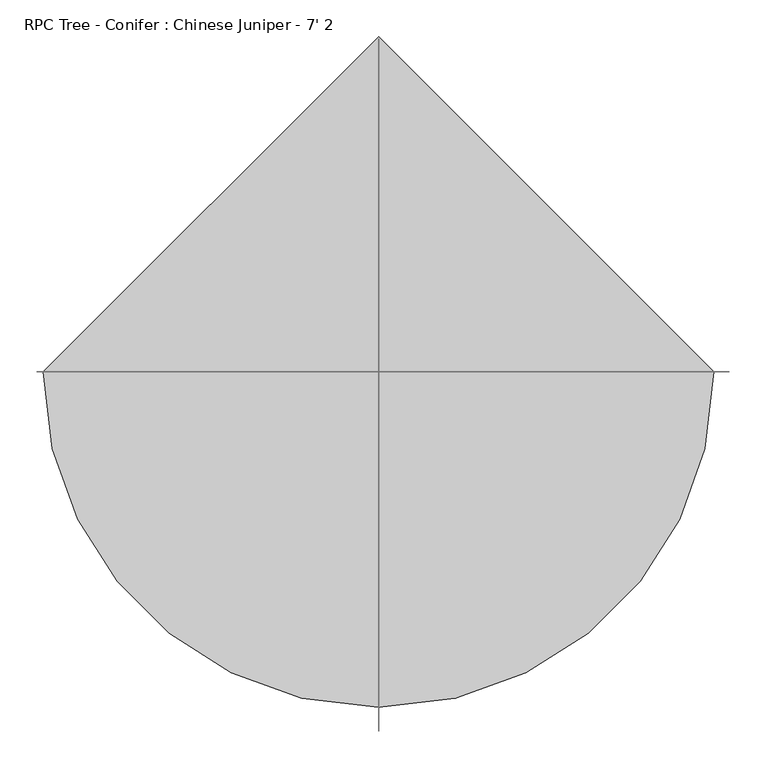
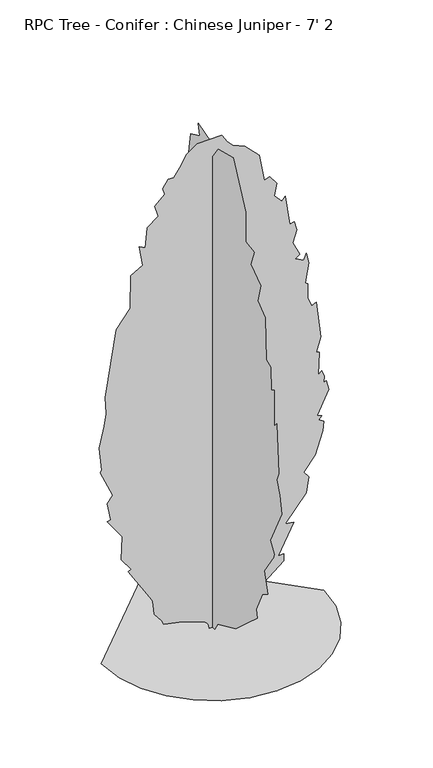
"""IFC4 building model written with IfcOpenShell, lengths in millimetres: geographic element geometry, RPC Tree - Conifer : Chinese Juniper - 7' 2."""

from ifc_helpers import new_model, si_unit, origin, place, context, project, spatial, triangles, source, transform, mapped, element, save


def rpc_tree_conifer_chinese_juniper_7_2_1b9786cd(model_context):
    return source(origin(), model_context, "Body", "Tessellation", [
        triangles([(-14.517647, 6e-07, 1.3e-06), (-18.0071097, -3e-07, 17.9396969), (-27.4223632, -6e-07, 30.3914521), (-123.5685295, 1.5e-06, 65.7757953), (-201.676062, 3.9e-06, 82.3498608), (-209.1624873, 3.1e-06, 101.0656516), (-239.326362, 2.1e-06, 139.6788561), (-246.5945957, -1e-06, 198.3880905), (-257.8249785, -1.9e-06, 220.8470939), (-347.6599566, -6.4e-06, 363.0865585), (-336.0369015, -7.4e-06, 370.071561), (-375.7854927, -8.9e-06, 425.7942498), (-371.7570322, -1.5e-05, 524.6285151), (-433.7535387, -1.74e-05, 610.1379032), (-418.7802157, -1.83e-05, 613.8793173), (-433.1718882, -2.22e-05, 689.5207758), (-411.2922644, -2.49e-05, 718.6876728), (-463.6977139, -2.95e-05, 834.7279736), (-456.2123059, -3.02e-05, 842.2133451), (-467.4416714, -3.58e-05, 943.2777431), (-447.126705, -4.19e-05, 1031.4541197), (-437.4949891, -4.53e-05, 1081.7767748), (-441.2389466, -4.94e-05, 1152.8969976), (-396.3214485, -6.81e-05, 1433.6338589), (-340.174585, -7.5e-05, 1508.4981846), (-337.1392688, -8.35e-05, 1648.2265743), (-287.7691355, -8.74e-05, 1676.941246), (-302.7424948, -9.18e-05, 1763.0323574), (-277.1874594, -9.21e-05, 1748.371479), (-269.0543621, -9.76e-05, 1834.1525803), (-224.1350836, -0.0001015, 1867.8406403), (-239.107916, -0.0001038, 1916.5022049), (-197.9328675, -0.0001078, 1953.9342224), (-205.4192747, -0.000109, 1980.1369835), (-182.9602713, -0.000112, 2013.8251888), (-160.5012679, -0.000113, 2013.8251888), (-134.7328734, -0.0001161, 2047.2821583), (-108.898967, -0.0001202, 2095.8470718), (-62.5486394, -0.0001241, 2127.2339642), (37.1144179, -0.0001285, 2128.801165), (60.3458442, -0.0001273, 2092.4307106), (82.8048476, -0.000127, 2069.9720524), (132.737601, -0.0001279, 2048.8239246), (191.3566519, -0.0001268, 1987.6224277), (213.8156735, -0.0001209, 1871.5845978), (236.2746769, -0.0001223, 1879.070042), (263.6666277, -0.0001212, 1839.8828991), (254.989959, -0.0001178, 1789.2351185), (284.9366594, -0.0001171, 1755.5469131), (299.9074571, -0.0001186, 1770.5202724), (318.6248102, -0.0001119, 1643.2505699), (337.3395836, -0.0001129, 1646.9946728), (347.517378, -0.0001111, 1609.9130699), (330.7888933, -0.0001074, 1559.0291119), (359.7983145, -0.000105, 1497.2687828), (340.1843954, -0.0001034, 1485.5084541), (374.7716738, -0.0001038, 1467.3220642), (386.0010392, -0.0001059, 1493.5248253), (397.230441, -0.0001037, 1448.6072182), (382.2596251, -9.81e-05, 1366.2577389), (393.0673594, -9.81e-05, 1357.3651131), (391.5662155, -9.44e-05, 1296.562429), (408.4598064, -9.28e-05, 1257.7053532), (427.1771233, -9.41e-05, 1265.1907974), (445.8918966, -8.55e-05, 1107.9794632), (427.1771233, -8.11e-05, 1048.0886421), (438.8332068, -8.14e-05, 1044.1287821), (434.6625312, -7.54e-05, 947.0217007), (449.6358905, -7.68e-05, 958.2511024), (460.8652559, -7.57e-05, 932.0483414), (457.1212984, -7.4e-05, 905.8481964), (468.3506639, -7.47e-05, 909.5896105), (479.5800293, -7.27e-05, 868.4161062), (430.9185737, -6.48e-05, 771.0931223), (449.6358905, -6.52e-05, 763.6077507), (438.4064887, -6.38e-05, 748.6343914), (457.1212984, -6.39e-05, 737.4049896), (453.1842567, -6.13e-05, 697.0620306), (423.4331657, -5.44e-05, 602.6499518), (374.7716738, -4.87e-05, 542.7590944), (397.230441, -4.81e-05, 516.5563697), (384.9545551, -4.37e-05, 451.166393), (299.9074571, -3.36e-05, 344.3717488), (333.5981332, -3.49e-05, 340.6277913), (269.9633001, -2.47e-05, 217.1038994), (292.4220673, -2.57e-05, 217.1038994), (292.4220673, -2.39e-05, 187.1584707), (127.7223548, -8.7e-06, 52.4044321), (127.7223548, -9.8e-06, 71.1202274), (15.4277284, -7e-07, 0.0), (0.1966721, 13.7891713, 0.00013), (0.1966737, 34.4811189, 14.2963339), (0.1966762, 77.4229995, 29.9456808), (0.1966783, 178.488651, 67.3772736), (0.1966827, 230.8930831, 116.0384931), (0.1966819, 208.4340797, 119.7817057), (0.1966904, 288.5449239, 235.2565704), (0.1966918, 264.5824875, 291.9663175), (0.196695, 331.9587347, 389.2892833), (0.1966967, 324.4733268, 434.2067814), (0.1967014, 373.1322753, 494.0976388), (0.1967052, 389.4924685, 565.7309481), (0.1967041, 380.6202267, 640.0820784), (0.1967106, 440.5110841, 729.9170746), (0.1967147, 444.2524981, 819.7546143), (0.196717, 422.6319428, 893.2725832), (0.1967196, 455.4818636, 1010.6565519), (0.19672, 425.5377248, 1051.8300562), (0.1967236, 388.1056346, 1171.611771), (0.1967244, 414.3083593, 1253.9613956), (0.1967283, 384.3616407, 1373.7430378), (0.1967298, 346.932094, 1444.8632607), (0.1967315, 328.2147772, 1594.5917667), (0.19673, 305.75601, 1583.362365), (0.1967359, 305.75601, 1718.1148956), (0.1967344, 260.8385118, 1729.3441521), (0.1967329, 237.0752094, 1809.303661), (0.1967352, 223.406676, 1875.3287006), (0.1967352, 178.488651, 1920.2461624), (0.1967401, 156.0296476, 2055.0011639), (0.1967346, 92.3955867, 2084.9454117), (0.1967371, 102.0598133, 2133.1292439), (0.1967319, 11.3487565, 2104.2112415), (0.1967329, 6.3027505, 2040.0278046), (0.1967297, -38.6152347, 2103.6627285), (0.1967262, -147.1670527, 2133.606831), (0.1967183, -237.0033388, 1950.1902649), (0.1967127, -237.0033388, 1822.9231785), (0.1967097, -296.2055936, 1812.3847229), (0.1967078, -270.691199, 1744.3175114), (0.1967065, -342.8426634, 1695.0642677), (0.196704, -323.0966666, 1617.050425), (0.1966999, -375.4995727, 1575.8744499), (0.1966957, -382.9874877, 1396.2018414), (0.1966938, -413.5488853, 1383.1639744), (0.1966894, -416.6756204, 1283.9081142), (0.196689, -439.1343876, 1298.8788574), (0.1966862, -439.1343876, 1141.6675959), (0.1966823, -457.849161, 1164.1263994), (0.1966765, -472.8225203, 954.5096884), (0.1966757, -456.5690065, 918.855542), (0.1966723, -480.3104716, 864.672076), (0.1966725, -491.5398371, 789.8078957), (0.1966689, -412.9316628, 628.8526766), (0.1966658, -439.1343876, 583.9351785), (0.1966692, -436.9195155, 568.0778978), (0.1966679, -368.0141647, 467.8974212), (0.1966629, -394.2168895, 381.8038754), (0.1966636, -353.0408054, 355.6011506), (0.1966655, -311.8672648, 265.7661362), (0.1966637, -319.3526728, 232.0767318), (0.196664, -244.4894916, 164.6997216), (0.1966643, -165.8828434, 93.5794897), (0.1966675, -34.8715179, 33.6886368), (0.1966708, -16.1562041, 0.0001282), (-457.9674314, 0.0, 0.0001492), (-445.8541446, -104.9808196, 0.0001424), (-411.358285, -201.3891246, 0.0001352), (-357.2408761, -286.4621113, 0.0001277), (-286.2654482, -357.4375574, 0.0001204), (-201.1924614, -411.5549664, 0.0001134), (-104.7841473, -446.0508259, 0.0001072), (0.1966917, -458.1641127, 0.0001019), (105.1774918, -446.0508259, 9.8e-05), (201.5857877, -411.5549664, 9.58e-05), (286.6587745, -357.4375574, 9.54e-05), (357.6342387, -286.4621113, 9.65e-05), (411.7516477, -201.3888702, 9.92e-05), (446.2475072, -104.9808196, 0.0001034), (458.360794, 4.01e-05, 0.0001092), (0.1966112, 458.1641127, 0.0001565)], [[57, 58, 59], [27, 28, 29], [87, 88, 89], [49, 50, 51], [13, 14, 15], [83, 84, 85], [74, 75, 76], [63, 64, 65], [68, 69, 70], [71, 72, 73], [9, 10, 11], [85, 86, 87], [85, 87, 89], [51, 52, 53], [54, 55, 56], [90, 1, 2], [66, 67, 68], [45, 46, 47], [17, 18, 19], [68, 70, 71], [45, 47, 48], [31, 32, 33], [76, 77, 78], [89, 90, 2], [89, 2, 3], [57, 59, 60], [51, 53, 54], [25, 26, 27], [39, 40, 41], [56, 57, 60], [71, 73, 74], [34, 35, 36], [33, 34, 36], [4, 5, 6], [60, 61, 62], [80, 81, 82], [38, 39, 41], [37, 38, 41], [37, 41, 42], [29, 30, 31], [15, 16, 17], [36, 37, 42], [33, 36, 42], [31, 33, 42], [31, 42, 43], [31, 43, 44], [31, 44, 45], [29, 31, 45], [29, 45, 48], [27, 29, 48], [25, 27, 48], [25, 48, 49], [25, 49, 51], [25, 51, 54], [25, 54, 56], [25, 56, 60], [25, 60, 62], [24, 25, 62], [23, 24, 62], [22, 23, 62], [22, 62, 63], [22, 63, 65], [22, 65, 66], [22, 66, 68], [21, 22, 68], [20, 21, 68], [19, 20, 68], [17, 19, 68], [17, 68, 71], [17, 71, 74], [15, 17, 74], [13, 15, 74], [13, 74, 76], [13, 76, 78], [13, 78, 79], [13, 79, 80], [12, 13, 80], [11, 12, 80], [9, 11, 80], [9, 80, 82], [9, 82, 83], [9, 83, 85], [9, 85, 89], [9, 89, 3], [9, 3, 4], [8, 9, 4], [8, 4, 6], [7, 8, 6], [138, 139, 140], [94, 95, 96], [136, 137, 138], [121, 122, 123], [112, 113, 114], [128, 129, 130], [121, 123, 124], [125, 126, 127], [124, 125, 127], [114, 115, 116], [147, 148, 149], [130, 131, 132], [124, 127, 128], [134, 135, 136], [154, 155, 91], [154, 91, 92], [150, 151, 152], [96, 97, 98], [119, 120, 121], [119, 121, 124], [119, 124, 128], [118, 119, 128], [117, 118, 128], [116, 117, 128], [116, 128, 130], [114, 116, 130], [114, 130, 132], [112, 114, 132], [112, 132, 133], [112, 133, 134], [112, 134, 136], [111, 112, 136], [110, 111, 136], [109, 110, 136], [109, 136, 138], [109, 138, 140], [109, 140, 141], [108, 109, 141], [107, 108, 141], [106, 107, 141], [105, 106, 141], [104, 105, 141], [103, 104, 141], [103, 141, 142], [103, 142, 143], [103, 143, 144], [102, 103, 144], [101, 102, 144], [100, 101, 144], [100, 144, 145], [100, 145, 146], [100, 146, 147], [100, 147, 149], [100, 149, 150], [100, 150, 152], [100, 152, 153], [100, 153, 154], [99, 100, 154], [98, 99, 154], [96, 98, 154], [96, 154, 92], [96, 92, 93], [96, 93, 94], [170, 171, 156], [169, 170, 156], [169, 156, 157], [168, 169, 157], [168, 157, 158], [168, 158, 159], [167, 168, 159], [166, 167, 159], [166, 159, 160], [166, 160, 161], [166, 161, 162], [166, 162, 163], [166, 163, 164], [166, 164, 165]], closed=False),
    ])


if __name__ == "__main__":
    model = new_model("IFC4")
    model_context = context("Model", 3, world=origin())
    ifc_project = project(units=[si_unit("LENGTHUNIT", "METRE", prefix="MILLI")], contexts=[model_context])
    site = spatial("IfcSite", under=ifc_project)
    building = spatial("IfcBuilding", under=site)
    placement = place(None, origin())
    rpc_tree_conifer_chinese_juniper_7_2_shape = rpc_tree_conifer_chinese_juniper_7_2_1b9786cd(model_context)
    element("IfcGeographicElement", 1, ObjectType="RPC Tree - Conifer : Chinese Juniper - 7' 2", at=placement, inside=building, context=model_context, shape_type="MappedRepresentation", body=[
        mapped(rpc_tree_conifer_chinese_juniper_7_2_shape, transform((0.0, 0.0, 0.0), x_axis=(1.0, 0.0, 0.0), y_axis=(0.0, 1.0, 0.0), z_axis=(0.0, 0.0, 1.0))),
    ])
    save(model, "model.ifc")

# Revit data of these elements
# Type "RPC Tree - Conifer : Chinese Juniper - 7' 2"
#   built-in parameter 1005198 = "{2, 15},{39, RPC-16-FUM3-UUQ0-UBF0-N000-ST1L-LVER-AU},{1, 0},{1, 0},{2, 35},{1, 8},{5, Color},{1, 0},{1, 0},{3, 0.8},{3, 0.8},{3, 0.8},{1, 8},{7, BBoxMin},{1, 0},{1, 0},{1, 0},{1, 0},{1, 0},{1, 8},{7, BBoxMax},{1, 0},{1, 0},{1, 0},{1, 0},{1, 0},{2, 11},{9, RPCTypeId},{1, 0},{1, 0},{39, RPC-16-FUM3-UUQ0-UBF0-N000-ST1L-LVER-AU},{1, 6},{14, RPCPlantHeight},{1, 0},{1, 0},{1, 7},{2, 11},{7, keyword},{1, 0},{1, 0},{96, :Geometry:RPC:Chinese Juniper:juniperus chinensis:chinese:juniper:cupressaceae:conifer:evergreen},{2, 11},{8, category},{1, 0},{1, 0},{16, :Trees [General]},{2, 11},{12, LocalizedUID},{1, 0},{1, 0},{15, Chinese Juniper},{2, 14},{6, Height},{1, 0},{1, 0},{1, 7},{1, 2},{16, Cast Reflections},{1, 0},{1, 0},{1, 0},{1, 2},{12, Cast Shadows},{1, 0},{1, 0},{1, 1},{1, 2},{9, Lock View},{1, 0},{1, 0},{1, 0},{1, 4},{5, ViewC},{1, 0},{1, 0},{1, 0},{2, 11},{20, AdvancedUIDefinition},{1, 0},{1, 0},{0, },{2, 11},{10, AssetLibID},{1, 0},{1, 0},{36, 4D3F6E72-3F99-4203-98E9-AF80B3C7A7A4},{2, 11},{10, BaseSchema},{1, 0},{1, 0},{9, RPCSchema},{2, 11},{12, ExchangeGUID},{1, 0},{1, 0},{0, },{1, 2},{6, Hidden},{1, 0},{1, 0},{1, 0},{1, 4},{11, RPCCategory},{1, 0},{1, 0},{1, 0},{2, 11},{8, RPCImage},{1, 0},{1, 0},{0, },{1, 4},{13, SchemaVersion},{1, 0},{1, 0},{1, 4},{2, 11},{12, UIDefinition},{1, 0},{1, 0},{0, },{2, 11},{6, UIName},{1, 0},{1, 0},{39, RPC-16-FUM3-UUQ0-UBF0-N000-ST1L-LVER-AU},{2, 11},{11, VersionGUID},{1, 0},{1, 0},{9, RPCSchema},{2, 11},{9, assettype},{1, 0},{1, 0},{11, RPCGeometry},{2, 11},{11, description},{1, 0},{1, 0},{0, },{2, 11},{9, localname},{1, 0},{1, 0},{3, RPC},{2, 11},{9, localtype},{1, 0},{1, 0},{3, RPC},{1, 4},{8, revision},{1, 0},{1, 0},{1, 1},{2, 11},{9, thumbnail},{1, 0},{1, 0},{0, },{1, 4},{7, version},{1, 0},{1, 0},{1, 1},{1, 2},{20, RPC_Cast Reflections},{1, 0},{1, 0},{1, 1},{1, 2},{16, RPC_Cast Shadows},{1, 0},{1, 0},{1, 1},{1, 2},{13, RPC_Lock View},{1, 0},{1, 0},{1, 0},{1, 4},{9, RPC_ViewC},{1, 0},{1, 0},{1, 0},{21, assetlibrary_base.fbx},{1, 5},"
#   built-in parameter 1005195 = "RPC-16-FUM3-UUQ0-UBF0-N000-ST1L-LVER-AU"
#   Type Comments = "Chinese Juniper"
#   Assembly Code = "G2050500"
#   Height = 7' - 0"
#   Description = (empty or 0)
#   Default Elevation = 0
